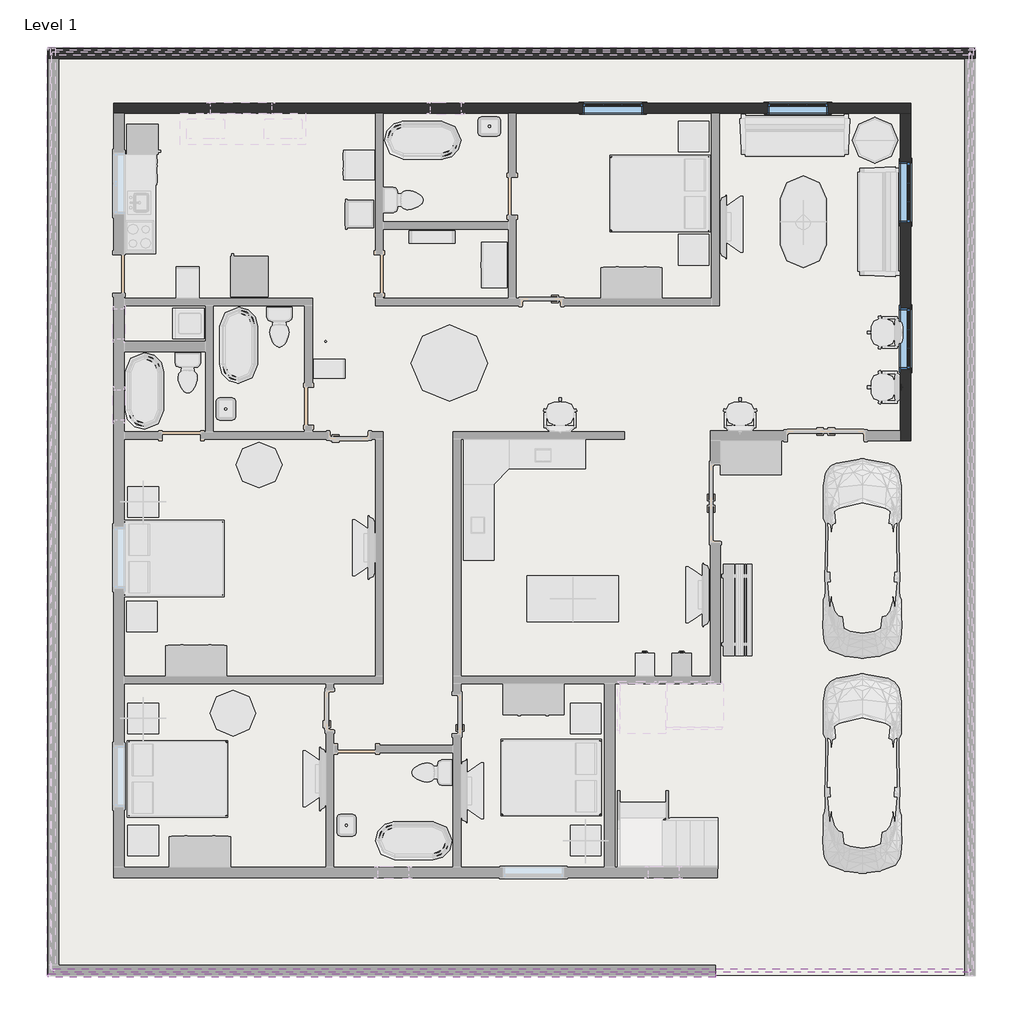
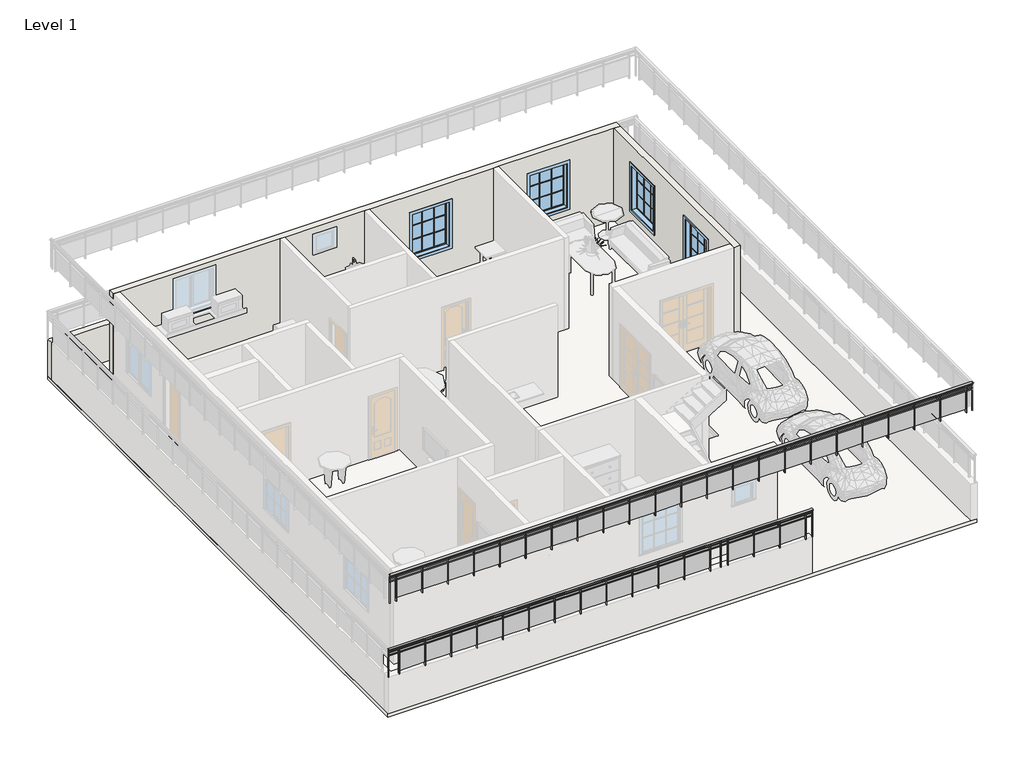
# One storey, part 2 of 6: 4 windows, 3 walls, 2 railings, 1 slab.
"""IFC4 building model written with IfcOpenShell, lengths in millimetres."""

from ifc_helpers import new_model, si_unit, point, frame, origin, place, context, project, spatial, polyline, ellipse_curve, trimmed, outline, extrude, faceted_brep, transform, mapped, element, save
from ifc_brep_helpers import plane_surface, extruded_surface, advanced_brep
from components import window_cfa1ffdd

model = new_model("IFC4")

# Units and contexts
model_context = context("Model", 3, world=origin())
ifc_project = project(units=[si_unit("LENGTHUNIT", "METRE", prefix="MILLI")], contexts=[model_context])

# Site, building, storey
site = spatial("IfcSite", under=ifc_project)
building = spatial("IfcBuilding", under=site)
storey = spatial("IfcBuildingStorey", under=building, Name="Level 1", Elevation=0.0)

# Railings
placement = place(None, origin())
element("IfcRailing", 1, ObjectType="Glass Panel - Bottom Fill", at=placement, inside=storey, context=model_context, shape_type="SolidModel", body=[
    advanced_brep(
    [(-7889.7402326, -4452.2366944, 2133.6), (-7889.7402326, -4528.4366944, 2133.6), (5419.8597674, -4452.2366944, 2133.6), (5419.8597674, -4528.4366944, 2133.6)],
    [
        (0, 1, ellipse_curve(frame((-7889.7402326, -4490.3366944, 2133.6), z_axis=(-1.0, 0.0, 0.0), x_axis=(0.0, -1.0, 0.0)), 38.1, 28.575)),
        (1, 0, ellipse_curve(frame((-7889.7402326, -4490.3366944, 2133.6), z_axis=(-1.0, 0.0, 0.0), x_axis=(0.0, -1.0, 0.0)), 38.1, 28.575)),
        (2, 3, ellipse_curve(frame((5419.8597674, -4490.3366944, 2133.6), z_axis=(1.0, 0.0, 0.0), x_axis=(0.0, -1.0, 0.0)), 38.1, 28.575)),
        (3, 2, ellipse_curve(frame((5419.8597674, -4490.3366944, 2133.6), z_axis=(1.0, 0.0, 0.0), x_axis=(0.0, -1.0, 0.0)), 38.1, 28.575)),
        (0, 2),
        (3, 1),
    ],
    [
        plane_surface(frame((-7889.7402326, -4490.3366944, 2133.6), z_axis=(-1.0, 0.0, 0.0), x_axis=(0.0, 1.0, 0.0))),
        plane_surface(frame((5419.8597674, -4490.3366944, 2133.6), z_axis=(1.0, 0.0, 0.0), x_axis=(0.0, 1.0, 0.0))),
        extruded_surface(trimmed(ellipse_curve(frame((5419.8597674, -4490.3366944, 2133.6), z_axis=(-1.0, 0.0, 0.0), x_axis=(0.0, -1.0, 0.0)), 38.1, 28.575), [point((5419.8597674, -4452.2366944, 2133.6))], [point((5419.8597674, -4528.4366944, 2133.6))], True, "CARTESIAN"), (-13309.6, 0.0, 0.0), 13309.6),
        extruded_surface(trimmed(ellipse_curve(frame((5419.8597674, -4490.3366944, 2133.6), z_axis=(-1.0, 0.0, 0.0), x_axis=(0.0, -1.0, 0.0)), 38.1, 28.575), [point((5419.8597674, -4528.4366944, 2133.6))], [point((5419.8597674, -4452.2366944, 2133.6))], True, "CARTESIAN"), (-13309.6, 0.0, 0.0), 13309.6),
    ],
    [
        (0, [[1, 2]]),
        (1, [[3, 4]]),
        (2, [[-1, 5, -4, 6]]),
        (3, [[-2, -6, -3, -5]]),
    ],
),
    extrude(outline(polyline([(-7889.7402326, -4503.0366944), (-7889.7402326, -4477.6366944), (5419.8597674, -4477.6366944), (5419.8597674, -4503.0366944), (-7889.7402326, -4503.0366944)])), frame((0.0, 0.0, 2019.3), z_axis=(0.0, 0.0, 1.0), x_axis=(1.0, 0.0, 0.0)), (0.0, 0.0, 1.0), 25.4),
    extrude(outline(polyline([(-7889.7402326, -4503.0366944), (-7889.7402326, -4477.6366944), (5419.8597674, -4477.6366944), (5419.8597674, -4503.0366944), (-7889.7402326, -4503.0366944)])), frame((0.0, 0.0, 1917.7), z_axis=(0.0, 0.0, 1.0), x_axis=(1.0, 0.0, 0.0)), (0.0, 0.0, 1.0), 25.4),
    extrude(outline(polyline([(5197.6097674, -4515.7366944), (5197.6097674, -4464.9366944), (5210.3097674, -4464.9366944), (5210.3097674, -4515.7366944), (5197.6097674, -4515.7366944)])), frame((0.0, 0.0, 1219.2), z_axis=(0.0, 0.0, 1.0), x_axis=(1.0, 0.0, 0.0)), (0.0, 0.0, 1.0), 885.6788223),
    extrude(outline(polyline([(4391.1597674, -4483.8015374), (5203.9597674, -4483.8015374), (5203.9597674, -4490.1515374), (4391.1597674, -4490.1515374), (4391.1597674, -4483.8015374)])), frame((0.0, 0.0, 1320.8), z_axis=(0.0, 0.0, 1.0), x_axis=(1.0, 0.0, 0.0)), (0.0, 0.0, 1.0), 596.9),
    extrude(outline(polyline([(4384.8097674, -4515.7366944), (4384.8097674, -4464.9366944), (4397.5097674, -4464.9366944), (4397.5097674, -4515.7366944), (4384.8097674, -4515.7366944)])), frame((0.0, 0.0, 1219.2), z_axis=(0.0, 0.0, 1.0), x_axis=(1.0, 0.0, 0.0)), (0.0, 0.0, 1.0), 885.6788223),
    extrude(outline(polyline([(3578.3597674, -4483.8015374), (4391.1597674, -4483.8015374), (4391.1597674, -4490.1515374), (3578.3597674, -4490.1515374), (3578.3597674, -4483.8015374)])), frame((0.0, 0.0, 1320.8), z_axis=(0.0, 0.0, 1.0), x_axis=(1.0, 0.0, 0.0)), (0.0, 0.0, 1.0), 596.9),
    extrude(outline(polyline([(3572.0097674, -4515.7366944), (3572.0097674, -4464.9366944), (3584.7097674, -4464.9366944), (3584.7097674, -4515.7366944), (3572.0097674, -4515.7366944)])), frame((0.0, 0.0, 1219.2), z_axis=(0.0, 0.0, 1.0), x_axis=(1.0, 0.0, 0.0)), (0.0, 0.0, 1.0), 885.6788223),
    extrude(outline(polyline([(2765.5597674, -4483.8015374), (3578.3597674, -4483.8015374), (3578.3597674, -4490.1515374), (2765.5597674, -4490.1515374), (2765.5597674, -4483.8015374)])), frame((0.0, 0.0, 1320.8), z_axis=(0.0, 0.0, 1.0), x_axis=(1.0, 0.0, 0.0)), (0.0, 0.0, 1.0), 596.9),
    extrude(outline(polyline([(2759.2097674, -4515.7366944), (2759.2097674, -4464.9366944), (2771.9097674, -4464.9366944), (2771.9097674, -4515.7366944), (2759.2097674, -4515.7366944)])), frame((0.0, 0.0, 1219.2), z_axis=(0.0, 0.0, 1.0), x_axis=(1.0, 0.0, 0.0)), (0.0, 0.0, 1.0), 885.6788223),
    extrude(outline(polyline([(2200.4097674, -4515.7366944), (2200.4097674, -4464.9366944), (2213.1097674, -4464.9366944), (2213.1097674, -4515.7366944), (2200.4097674, -4515.7366944)])), frame((0.0, 0.0, 1219.2), z_axis=(0.0, 0.0, 1.0), x_axis=(1.0, 0.0, 0.0)), (0.0, 0.0, 1.0), 885.6788223),
    extrude(outline(polyline([(1393.9597674, -4483.8015374), (2206.7597674, -4483.8015374), (2206.7597674, -4490.1515374), (1393.9597674, -4490.1515374), (1393.9597674, -4483.8015374)])), frame((0.0, 0.0, 1320.8), z_axis=(0.0, 0.0, 1.0), x_axis=(1.0, 0.0, 0.0)), (0.0, 0.0, 1.0), 596.9),
    extrude(outline(polyline([(1387.6097674, -4515.7366944), (1387.6097674, -4464.9366944), (1400.3097674, -4464.9366944), (1400.3097674, -4515.7366944), (1387.6097674, -4515.7366944)])), frame((0.0, 0.0, 1219.2), z_axis=(0.0, 0.0, 1.0), x_axis=(1.0, 0.0, 0.0)), (0.0, 0.0, 1.0), 885.6788223),
    extrude(outline(polyline([(581.1597674, -4483.8015374), (1393.9597674, -4483.8015374), (1393.9597674, -4490.1515374), (581.1597674, -4490.1515374), (581.1597674, -4483.8015374)])), frame((0.0, 0.0, 1320.8), z_axis=(0.0, 0.0, 1.0), x_axis=(1.0, 0.0, 0.0)), (0.0, 0.0, 1.0), 596.9),
    extrude(outline(polyline([(574.8097674, -4515.7366944), (574.8097674, -4464.9366944), (587.5097674, -4464.9366944), (587.5097674, -4515.7366944), (574.8097674, -4515.7366944)])), frame((0.0, 0.0, 1219.2), z_axis=(0.0, 0.0, 1.0), x_axis=(1.0, 0.0, 0.0)), (0.0, 0.0, 1.0), 885.6788223),
    extrude(outline(polyline([(-231.6402326, -4483.8015374), (581.1597674, -4483.8015374), (581.1597674, -4490.1515374), (-231.6402326, -4490.1515374), (-231.6402326, -4483.8015374)])), frame((0.0, 0.0, 1320.8), z_axis=(0.0, 0.0, 1.0), x_axis=(1.0, 0.0, 0.0)), (0.0, 0.0, 1.0), 596.9),
    extrude(outline(polyline([(-237.9902326, -4515.7366944), (-237.9902326, -4464.9366944), (-225.2902326, -4464.9366944), (-225.2902326, -4515.7366944), (-237.9902326, -4515.7366944)])), frame((0.0, 0.0, 1219.2), z_axis=(0.0, 0.0, 1.0), x_axis=(1.0, 0.0, 0.0)), (0.0, 0.0, 1.0), 885.6788223),
    extrude(outline(polyline([(-1044.4402326, -4483.8015374), (-231.6402326, -4483.8015374), (-231.6402326, -4490.1515374), (-1044.4402326, -4490.1515374), (-1044.4402326, -4483.8015374)])), frame((0.0, 0.0, 1320.8), z_axis=(0.0, 0.0, 1.0), x_axis=(1.0, 0.0, 0.0)), (0.0, 0.0, 1.0), 596.9),
    extrude(outline(polyline([(-1050.7902326, -4515.7366944), (-1050.7902326, -4464.9366944), (-1038.0902326, -4464.9366944), (-1038.0902326, -4515.7366944), (-1050.7902326, -4515.7366944)])), frame((0.0, 0.0, 1219.2), z_axis=(0.0, 0.0, 1.0), x_axis=(1.0, 0.0, 0.0)), (0.0, 0.0, 1.0), 885.6788223),
    extrude(outline(polyline([(-1857.2402326, -4483.8015374), (-1044.4402326, -4483.8015374), (-1044.4402326, -4490.1515374), (-1857.2402326, -4490.1515374), (-1857.2402326, -4483.8015374)])), frame((0.0, 0.0, 1320.8), z_axis=(0.0, 0.0, 1.0), x_axis=(1.0, 0.0, 0.0)), (0.0, 0.0, 1.0), 596.9),
    extrude(outline(polyline([(-1863.5902326, -4515.7366944), (-1863.5902326, -4464.9366944), (-1850.8902326, -4464.9366944), (-1850.8902326, -4515.7366944), (-1863.5902326, -4515.7366944)])), frame((0.0, 0.0, 1219.2), z_axis=(0.0, 0.0, 1.0), x_axis=(1.0, 0.0, 0.0)), (0.0, 0.0, 1.0), 885.6788223),
    extrude(outline(polyline([(-2670.0402326, -4483.8015374), (-1857.2402326, -4483.8015374), (-1857.2402326, -4490.1515374), (-2670.0402326, -4490.1515374), (-2670.0402326, -4483.8015374)])), frame((0.0, 0.0, 1320.8), z_axis=(0.0, 0.0, 1.0), x_axis=(1.0, 0.0, 0.0)), (0.0, 0.0, 1.0), 596.9),
    extrude(outline(polyline([(-2676.3902326, -4515.7366944), (-2676.3902326, -4464.9366944), (-2663.6902326, -4464.9366944), (-2663.6902326, -4515.7366944), (-2676.3902326, -4515.7366944)])), frame((0.0, 0.0, 1219.2), z_axis=(0.0, 0.0, 1.0), x_axis=(1.0, 0.0, 0.0)), (0.0, 0.0, 1.0), 885.6788223),
    extrude(outline(polyline([(-3482.8402326, -4483.8015374), (-2670.0402326, -4483.8015374), (-2670.0402326, -4490.1515374), (-3482.8402326, -4490.1515374), (-3482.8402326, -4483.8015374)])), frame((0.0, 0.0, 1320.8), z_axis=(0.0, 0.0, 1.0), x_axis=(1.0, 0.0, 0.0)), (0.0, 0.0, 1.0), 596.9),
    extrude(outline(polyline([(-3489.1902326, -4515.7366944), (-3489.1902326, -4464.9366944), (-3476.4902326, -4464.9366944), (-3476.4902326, -4515.7366944), (-3489.1902326, -4515.7366944)])), frame((0.0, 0.0, 1219.2), z_axis=(0.0, 0.0, 1.0), x_axis=(1.0, 0.0, 0.0)), (0.0, 0.0, 1.0), 885.6788223),
    extrude(outline(polyline([(-4295.6402326, -4483.8015374), (-3482.8402326, -4483.8015374), (-3482.8402326, -4490.1515374), (-4295.6402326, -4490.1515374), (-4295.6402326, -4483.8015374)])), frame((0.0, 0.0, 1320.8), z_axis=(0.0, 0.0, 1.0), x_axis=(1.0, 0.0, 0.0)), (0.0, 0.0, 1.0), 596.9),
    extrude(outline(polyline([(-4301.9902326, -4515.7366944), (-4301.9902326, -4464.9366944), (-4289.2902326, -4464.9366944), (-4289.2902326, -4515.7366944), (-4301.9902326, -4515.7366944)])), frame((0.0, 0.0, 1219.2), z_axis=(0.0, 0.0, 1.0), x_axis=(1.0, 0.0, 0.0)), (0.0, 0.0, 1.0), 885.6788223),
    extrude(outline(polyline([(-5108.4402326, -4483.8015374), (-4295.6402326, -4483.8015374), (-4295.6402326, -4490.1515374), (-5108.4402326, -4490.1515374), (-5108.4402326, -4483.8015374)])), frame((0.0, 0.0, 1320.8), z_axis=(0.0, 0.0, 1.0), x_axis=(1.0, 0.0, 0.0)), (0.0, 0.0, 1.0), 596.9),
    extrude(outline(polyline([(-5114.7902326, -4515.7366944), (-5114.7902326, -4464.9366944), (-5102.0902326, -4464.9366944), (-5102.0902326, -4515.7366944), (-5114.7902326, -4515.7366944)])), frame((0.0, 0.0, 1219.2), z_axis=(0.0, 0.0, 1.0), x_axis=(1.0, 0.0, 0.0)), (0.0, 0.0, 1.0), 885.6788223),
    extrude(outline(polyline([(-5921.2402326, -4483.8015374), (-5108.4402326, -4483.8015374), (-5108.4402326, -4490.1515374), (-5921.2402326, -4490.1515374), (-5921.2402326, -4483.8015374)])), frame((0.0, 0.0, 1320.8), z_axis=(0.0, 0.0, 1.0), x_axis=(1.0, 0.0, 0.0)), (0.0, 0.0, 1.0), 596.9),
    extrude(outline(polyline([(-5927.5902326, -4515.7366944), (-5927.5902326, -4464.9366944), (-5914.8902326, -4464.9366944), (-5914.8902326, -4515.7366944), (-5927.5902326, -4515.7366944)])), frame((0.0, 0.0, 1219.2), z_axis=(0.0, 0.0, 1.0), x_axis=(1.0, 0.0, 0.0)), (0.0, 0.0, 1.0), 885.6788223),
    extrude(outline(polyline([(-6734.0402326, -4483.8015374), (-5921.2402326, -4483.8015374), (-5921.2402326, -4490.1515374), (-6734.0402326, -4490.1515374), (-6734.0402326, -4483.8015374)])), frame((0.0, 0.0, 1320.8), z_axis=(0.0, 0.0, 1.0), x_axis=(1.0, 0.0, 0.0)), (0.0, 0.0, 1.0), 596.9),
    extrude(outline(polyline([(-6740.3902326, -4515.7366944), (-6740.3902326, -4464.9366944), (-6727.6902326, -4464.9366944), (-6727.6902326, -4515.7366944), (-6740.3902326, -4515.7366944)])), frame((0.0, 0.0, 1219.2), z_axis=(0.0, 0.0, 1.0), x_axis=(1.0, 0.0, 0.0)), (0.0, 0.0, 1.0), 885.6788223),
    extrude(outline(polyline([(-7546.8402326, -4483.8015374), (-6734.0402326, -4483.8015374), (-6734.0402326, -4490.1515374), (-7546.8402326, -4490.1515374), (-7546.8402326, -4483.8015374)])), frame((0.0, 0.0, 1320.8), z_axis=(0.0, 0.0, 1.0), x_axis=(1.0, 0.0, 0.0)), (0.0, 0.0, 1.0), 596.9),
    extrude(outline(polyline([(-7553.1902326, -4515.7366944), (-7553.1902326, -4464.9366944), (-7540.4902326, -4464.9366944), (-7540.4902326, -4515.7366944), (-7553.1902326, -4515.7366944)])), frame((0.0, 0.0, 1219.2), z_axis=(0.0, 0.0, 1.0), x_axis=(1.0, 0.0, 0.0)), (0.0, 0.0, 1.0), 885.6788223),
    extrude(outline(polyline([(2540.1347674, -4499.8616944), (2540.1347674, -4480.8116944), (2559.1847674, -4480.8116944), (2559.1847674, -4499.8616944), (2540.1347674, -4499.8616944)])), frame((0.0, 0.0, 1219.2), z_axis=(0.0, 0.0, 1.0), x_axis=(1.0, 0.0, 0.0)), (0.0, 0.0, 1.0), 885.6788223),
    extrude(outline(polyline([(5407.1597674, -4499.8616944), (5407.1597674, -4480.8116944), (5426.2097674, -4480.8116944), (5426.2097674, -4499.8616944), (5407.1597674, -4499.8616944)])), frame((0.0, 0.0, 1219.2), z_axis=(0.0, 0.0, 1.0), x_axis=(1.0, 0.0, 0.0)), (0.0, 0.0, 1.0), 885.6788223),
    extrude(outline(polyline([(-7896.0902326, -4499.8616944), (-7896.0902326, -4480.8116944), (-7877.0402326, -4480.8116944), (-7877.0402326, -4499.8616944), (-7896.0902326, -4499.8616944)])), frame((0.0, 0.0, 1219.2), z_axis=(0.0, 0.0, 1.0), x_axis=(1.0, 0.0, 0.0)), (0.0, 0.0, 1.0), 885.6788223),
])
element("IfcRailing", 2, ObjectType="Glass Panel - Bottom Fill", at=placement, inside=storey, context=model_context, shape_type="SolidModel", body=[
    advanced_brep(
    [(-7788.1402326, -4350.6366944, 4495.8), (-7788.1402326, -4426.8366944, 4495.8), (10499.8597674, -4350.6366944, 4495.8), (10499.8597674, -4426.8366944, 4495.8)],
    [
        (0, 1, ellipse_curve(frame((-7788.1402326, -4388.7366944, 4495.8), z_axis=(-1.0, 0.0, 0.0), x_axis=(0.0, -1.0, 0.0)), 38.1, 28.575)),
        (1, 0, ellipse_curve(frame((-7788.1402326, -4388.7366944, 4495.8), z_axis=(-1.0, 0.0, 0.0), x_axis=(0.0, -1.0, 0.0)), 38.1, 28.575)),
        (2, 3, ellipse_curve(frame((10499.8597674, -4388.7366944, 4495.8), z_axis=(1.0, 0.0, 0.0), x_axis=(0.0, -1.0, 0.0)), 38.1, 28.575)),
        (3, 2, ellipse_curve(frame((10499.8597674, -4388.7366944, 4495.8), z_axis=(1.0, 0.0, 0.0), x_axis=(0.0, -1.0, 0.0)), 38.1, 28.575)),
        (0, 2),
        (3, 1),
    ],
    [
        plane_surface(frame((-7788.1402326, -4388.7366944, 4495.8), z_axis=(-1.0, 0.0, 0.0), x_axis=(0.0, 1.0, 0.0))),
        plane_surface(frame((10499.8597674, -4388.7366944, 4495.8), z_axis=(1.0, 0.0, 0.0), x_axis=(0.0, 1.0, 0.0))),
        extruded_surface(trimmed(ellipse_curve(frame((10499.8597674, -4388.7366944, 4495.8), z_axis=(-1.0, 0.0, 0.0), x_axis=(0.0, -1.0, 0.0)), 38.1, 28.575), [point((10499.8597674, -4350.6366944, 4495.8))], [point((10499.8597674, -4426.8366944, 4495.8))], True, "CARTESIAN"), (-18288.0, 0.0, 0.0), 18288.0),
        extruded_surface(trimmed(ellipse_curve(frame((10499.8597674, -4388.7366944, 4495.8), z_axis=(-1.0, 0.0, 0.0), x_axis=(0.0, -1.0, 0.0)), 38.1, 28.575), [point((10499.8597674, -4426.8366944, 4495.8))], [point((10499.8597674, -4350.6366944, 4495.8))], True, "CARTESIAN"), (-18288.0, 0.0, 0.0), 18288.0),
    ],
    [
        (0, [[1, 2]]),
        (1, [[3, 4]]),
        (2, [[-1, 5, -4, 6]]),
        (3, [[-2, -6, -3, -5]]),
    ],
),
    extrude(outline(polyline([(-7788.1402326, -4401.4366944), (-7788.1402326, -4376.0366944), (10499.8597674, -4376.0366944), (10499.8597674, -4401.4366944), (-7788.1402326, -4401.4366944)])), frame((0.0, 0.0, 4381.5), z_axis=(0.0, 0.0, 1.0), x_axis=(1.0, 0.0, 0.0)), (0.0, 0.0, 1.0), 25.4),
    extrude(outline(polyline([(-7788.1402326, -4401.4366944), (-7788.1402326, -4376.0366944), (10499.8597674, -4376.0366944), (10499.8597674, -4401.4366944), (-7788.1402326, -4401.4366944)])), frame((0.0, 0.0, 4279.9), z_axis=(0.0, 0.0, 1.0), x_axis=(1.0, 0.0, 0.0)), (0.0, 0.0, 1.0), 25.4),
    extrude(outline(polyline([(10290.3097674, -4414.1366944), (10290.3097674, -4363.3366944), (10303.0097674, -4363.3366944), (10303.0097674, -4414.1366944), (10290.3097674, -4414.1366944)])), frame((0.0, 0.0, 3581.4), z_axis=(0.0, 0.0, 1.0), x_axis=(1.0, 0.0, 0.0)), (0.0, 0.0, 1.0), 885.6788223),
    extrude(outline(polyline([(9483.8597674, -4382.2015374), (10296.6597674, -4382.2015374), (10296.6597674, -4388.5515374), (9483.8597674, -4388.5515374), (9483.8597674, -4382.2015374)])), frame((0.0, 0.0, 3683.0), z_axis=(0.0, 0.0, 1.0), x_axis=(1.0, 0.0, 0.0)), (0.0, 0.0, 1.0), 596.9),
    extrude(outline(polyline([(9477.5097674, -4414.1366944), (9477.5097674, -4363.3366944), (9490.2097674, -4363.3366944), (9490.2097674, -4414.1366944), (9477.5097674, -4414.1366944)])), frame((0.0, 0.0, 3581.4), z_axis=(0.0, 0.0, 1.0), x_axis=(1.0, 0.0, 0.0)), (0.0, 0.0, 1.0), 885.6788223),
    extrude(outline(polyline([(8671.0597674, -4382.2015374), (9483.8597674, -4382.2015374), (9483.8597674, -4388.5515374), (8671.0597674, -4388.5515374), (8671.0597674, -4382.2015374)])), frame((0.0, 0.0, 3683.0), z_axis=(0.0, 0.0, 1.0), x_axis=(1.0, 0.0, 0.0)), (0.0, 0.0, 1.0), 596.9),
    extrude(outline(polyline([(8664.7097674, -4414.1366944), (8664.7097674, -4363.3366944), (8677.4097674, -4363.3366944), (8677.4097674, -4414.1366944), (8664.7097674, -4414.1366944)])), frame((0.0, 0.0, 3581.4), z_axis=(0.0, 0.0, 1.0), x_axis=(1.0, 0.0, 0.0)), (0.0, 0.0, 1.0), 885.6788223),
    extrude(outline(polyline([(7858.2597674, -4382.2015374), (8671.0597674, -4382.2015374), (8671.0597674, -4388.5515374), (7858.2597674, -4388.5515374), (7858.2597674, -4382.2015374)])), frame((0.0, 0.0, 3683.0), z_axis=(0.0, 0.0, 1.0), x_axis=(1.0, 0.0, 0.0)), (0.0, 0.0, 1.0), 596.9),
    extrude(outline(polyline([(7851.9097674, -4414.1366944), (7851.9097674, -4363.3366944), (7864.6097674, -4363.3366944), (7864.6097674, -4414.1366944), (7851.9097674, -4414.1366944)])), frame((0.0, 0.0, 3581.4), z_axis=(0.0, 0.0, 1.0), x_axis=(1.0, 0.0, 0.0)), (0.0, 0.0, 1.0), 885.6788223),
    extrude(outline(polyline([(7045.4597674, -4382.2015374), (7858.2597674, -4382.2015374), (7858.2597674, -4388.5515374), (7045.4597674, -4388.5515374), (7045.4597674, -4382.2015374)])), frame((0.0, 0.0, 3683.0), z_axis=(0.0, 0.0, 1.0), x_axis=(1.0, 0.0, 0.0)), (0.0, 0.0, 1.0), 596.9),
    extrude(outline(polyline([(7039.1097674, -4414.1366944), (7039.1097674, -4363.3366944), (7051.8097674, -4363.3366944), (7051.8097674, -4414.1366944), (7039.1097674, -4414.1366944)])), frame((0.0, 0.0, 3581.4), z_axis=(0.0, 0.0, 1.0), x_axis=(1.0, 0.0, 0.0)), (0.0, 0.0, 1.0), 885.6788223),
    extrude(outline(polyline([(6232.6597674, -4382.2015374), (7045.4597674, -4382.2015374), (7045.4597674, -4388.5515374), (6232.6597674, -4388.5515374), (6232.6597674, -4382.2015374)])), frame((0.0, 0.0, 3683.0), z_axis=(0.0, 0.0, 1.0), x_axis=(1.0, 0.0, 0.0)), (0.0, 0.0, 1.0), 596.9),
    extrude(outline(polyline([(6226.3097674, -4414.1366944), (6226.3097674, -4363.3366944), (6239.0097674, -4363.3366944), (6239.0097674, -4414.1366944), (6226.3097674, -4414.1366944)])), frame((0.0, 0.0, 3581.4), z_axis=(0.0, 0.0, 1.0), x_axis=(1.0, 0.0, 0.0)), (0.0, 0.0, 1.0), 885.6788223),
    extrude(outline(polyline([(5419.8597674, -4382.2015374), (6232.6597674, -4382.2015374), (6232.6597674, -4388.5515374), (5419.8597674, -4388.5515374), (5419.8597674, -4382.2015374)])), frame((0.0, 0.0, 3683.0), z_axis=(0.0, 0.0, 1.0), x_axis=(1.0, 0.0, 0.0)), (0.0, 0.0, 1.0), 596.9),
    extrude(outline(polyline([(5413.5097674, -4414.1366944), (5413.5097674, -4363.3366944), (5426.2097674, -4363.3366944), (5426.2097674, -4414.1366944), (5413.5097674, -4414.1366944)])), frame((0.0, 0.0, 3581.4), z_axis=(0.0, 0.0, 1.0), x_axis=(1.0, 0.0, 0.0)), (0.0, 0.0, 1.0), 885.6788223),
    extrude(outline(polyline([(4607.0597674, -4382.2015374), (5419.8597674, -4382.2015374), (5419.8597674, -4388.5515374), (4607.0597674, -4388.5515374), (4607.0597674, -4382.2015374)])), frame((0.0, 0.0, 3683.0), z_axis=(0.0, 0.0, 1.0), x_axis=(1.0, 0.0, 0.0)), (0.0, 0.0, 1.0), 596.9),
    extrude(outline(polyline([(4600.7097674, -4414.1366944), (4600.7097674, -4363.3366944), (4613.4097674, -4363.3366944), (4613.4097674, -4414.1366944), (4600.7097674, -4414.1366944)])), frame((0.0, 0.0, 3581.4), z_axis=(0.0, 0.0, 1.0), x_axis=(1.0, 0.0, 0.0)), (0.0, 0.0, 1.0), 885.6788223),
    extrude(outline(polyline([(3794.2597674, -4382.2015374), (4607.0597674, -4382.2015374), (4607.0597674, -4388.5515374), (3794.2597674, -4388.5515374), (3794.2597674, -4382.2015374)])), frame((0.0, 0.0, 3683.0), z_axis=(0.0, 0.0, 1.0), x_axis=(1.0, 0.0, 0.0)), (0.0, 0.0, 1.0), 596.9),
    extrude(outline(polyline([(3787.9097674, -4414.1366944), (3787.9097674, -4363.3366944), (3800.6097674, -4363.3366944), (3800.6097674, -4414.1366944), (3787.9097674, -4414.1366944)])), frame((0.0, 0.0, 3581.4), z_axis=(0.0, 0.0, 1.0), x_axis=(1.0, 0.0, 0.0)), (0.0, 0.0, 1.0), 885.6788223),
    extrude(outline(polyline([(2981.4597674, -4382.2015374), (3794.2597674, -4382.2015374), (3794.2597674, -4388.5515374), (2981.4597674, -4388.5515374), (2981.4597674, -4382.2015374)])), frame((0.0, 0.0, 3683.0), z_axis=(0.0, 0.0, 1.0), x_axis=(1.0, 0.0, 0.0)), (0.0, 0.0, 1.0), 596.9),
    extrude(outline(polyline([(2975.1097674, -4414.1366944), (2975.1097674, -4363.3366944), (2987.8097674, -4363.3366944), (2987.8097674, -4414.1366944), (2975.1097674, -4414.1366944)])), frame((0.0, 0.0, 3581.4), z_axis=(0.0, 0.0, 1.0), x_axis=(1.0, 0.0, 0.0)), (0.0, 0.0, 1.0), 885.6788223),
    extrude(outline(polyline([(2168.6597674, -4382.2015374), (2981.4597674, -4382.2015374), (2981.4597674, -4388.5515374), (2168.6597674, -4388.5515374), (2168.6597674, -4382.2015374)])), frame((0.0, 0.0, 3683.0), z_axis=(0.0, 0.0, 1.0), x_axis=(1.0, 0.0, 0.0)), (0.0, 0.0, 1.0), 596.9),
    extrude(outline(polyline([(2162.3097674, -4414.1366944), (2162.3097674, -4363.3366944), (2175.0097674, -4363.3366944), (2175.0097674, -4414.1366944), (2162.3097674, -4414.1366944)])), frame((0.0, 0.0, 3581.4), z_axis=(0.0, 0.0, 1.0), x_axis=(1.0, 0.0, 0.0)), (0.0, 0.0, 1.0), 885.6788223),
    extrude(outline(polyline([(1355.8597674, -4382.2015374), (2168.6597674, -4382.2015374), (2168.6597674, -4388.5515374), (1355.8597674, -4388.5515374), (1355.8597674, -4382.2015374)])), frame((0.0, 0.0, 3683.0), z_axis=(0.0, 0.0, 1.0), x_axis=(1.0, 0.0, 0.0)), (0.0, 0.0, 1.0), 596.9),
    extrude(outline(polyline([(1349.5097674, -4414.1366944), (1349.5097674, -4363.3366944), (1362.2097674, -4363.3366944), (1362.2097674, -4414.1366944), (1349.5097674, -4414.1366944)])), frame((0.0, 0.0, 3581.4), z_axis=(0.0, 0.0, 1.0), x_axis=(1.0, 0.0, 0.0)), (0.0, 0.0, 1.0), 885.6788223),
    extrude(outline(polyline([(543.0597674, -4382.2015374), (1355.8597674, -4382.2015374), (1355.8597674, -4388.5515374), (543.0597674, -4388.5515374), (543.0597674, -4382.2015374)])), frame((0.0, 0.0, 3683.0), z_axis=(0.0, 0.0, 1.0), x_axis=(1.0, 0.0, 0.0)), (0.0, 0.0, 1.0), 596.9),
    extrude(outline(polyline([(536.7097674, -4414.1366944), (536.7097674, -4363.3366944), (549.4097674, -4363.3366944), (549.4097674, -4414.1366944), (536.7097674, -4414.1366944)])), frame((0.0, 0.0, 3581.4), z_axis=(0.0, 0.0, 1.0), x_axis=(1.0, 0.0, 0.0)), (0.0, 0.0, 1.0), 885.6788223),
    extrude(outline(polyline([(-269.7402326, -4382.2015374), (543.0597674, -4382.2015374), (543.0597674, -4388.5515374), (-269.7402326, -4388.5515374), (-269.7402326, -4382.2015374)])), frame((0.0, 0.0, 3683.0), z_axis=(0.0, 0.0, 1.0), x_axis=(1.0, 0.0, 0.0)), (0.0, 0.0, 1.0), 596.9),
    extrude(outline(polyline([(-276.0902326, -4414.1366944), (-276.0902326, -4363.3366944), (-263.3902326, -4363.3366944), (-263.3902326, -4414.1366944), (-276.0902326, -4414.1366944)])), frame((0.0, 0.0, 3581.4), z_axis=(0.0, 0.0, 1.0), x_axis=(1.0, 0.0, 0.0)), (0.0, 0.0, 1.0), 885.6788223),
    extrude(outline(polyline([(-1082.5402326, -4382.2015374), (-269.7402326, -4382.2015374), (-269.7402326, -4388.5515374), (-1082.5402326, -4388.5515374), (-1082.5402326, -4382.2015374)])), frame((0.0, 0.0, 3683.0), z_axis=(0.0, 0.0, 1.0), x_axis=(1.0, 0.0, 0.0)), (0.0, 0.0, 1.0), 596.9),
    extrude(outline(polyline([(-1088.8902326, -4414.1366944), (-1088.8902326, -4363.3366944), (-1076.1902326, -4363.3366944), (-1076.1902326, -4414.1366944), (-1088.8902326, -4414.1366944)])), frame((0.0, 0.0, 3581.4), z_axis=(0.0, 0.0, 1.0), x_axis=(1.0, 0.0, 0.0)), (0.0, 0.0, 1.0), 885.6788223),
    extrude(outline(polyline([(-1895.3402326, -4382.2015374), (-1082.5402326, -4382.2015374), (-1082.5402326, -4388.5515374), (-1895.3402326, -4388.5515374), (-1895.3402326, -4382.2015374)])), frame((0.0, 0.0, 3683.0), z_axis=(0.0, 0.0, 1.0), x_axis=(1.0, 0.0, 0.0)), (0.0, 0.0, 1.0), 596.9),
    extrude(outline(polyline([(-1901.6902326, -4414.1366944), (-1901.6902326, -4363.3366944), (-1888.9902326, -4363.3366944), (-1888.9902326, -4414.1366944), (-1901.6902326, -4414.1366944)])), frame((0.0, 0.0, 3581.4), z_axis=(0.0, 0.0, 1.0), x_axis=(1.0, 0.0, 0.0)), (0.0, 0.0, 1.0), 885.6788223),
    extrude(outline(polyline([(-2708.1402326, -4382.2015374), (-1895.3402326, -4382.2015374), (-1895.3402326, -4388.5515374), (-2708.1402326, -4388.5515374), (-2708.1402326, -4382.2015374)])), frame((0.0, 0.0, 3683.0), z_axis=(0.0, 0.0, 1.0), x_axis=(1.0, 0.0, 0.0)), (0.0, 0.0, 1.0), 596.9),
    extrude(outline(polyline([(-2714.4902326, -4414.1366944), (-2714.4902326, -4363.3366944), (-2701.7902326, -4363.3366944), (-2701.7902326, -4414.1366944), (-2714.4902326, -4414.1366944)])), frame((0.0, 0.0, 3581.4), z_axis=(0.0, 0.0, 1.0), x_axis=(1.0, 0.0, 0.0)), (0.0, 0.0, 1.0), 885.6788223),
    extrude(outline(polyline([(-3520.9402326, -4382.2015374), (-2708.1402326, -4382.2015374), (-2708.1402326, -4388.5515374), (-3520.9402326, -4388.5515374), (-3520.9402326, -4382.2015374)])), frame((0.0, 0.0, 3683.0), z_axis=(0.0, 0.0, 1.0), x_axis=(1.0, 0.0, 0.0)), (0.0, 0.0, 1.0), 596.9),
    extrude(outline(polyline([(-3527.2902326, -4414.1366944), (-3527.2902326, -4363.3366944), (-3514.5902326, -4363.3366944), (-3514.5902326, -4414.1366944), (-3527.2902326, -4414.1366944)])), frame((0.0, 0.0, 3581.4), z_axis=(0.0, 0.0, 1.0), x_axis=(1.0, 0.0, 0.0)), (0.0, 0.0, 1.0), 885.6788223),
    extrude(outline(polyline([(-4333.7402326, -4382.2015374), (-3520.9402326, -4382.2015374), (-3520.9402326, -4388.5515374), (-4333.7402326, -4388.5515374), (-4333.7402326, -4382.2015374)])), frame((0.0, 0.0, 3683.0), z_axis=(0.0, 0.0, 1.0), x_axis=(1.0, 0.0, 0.0)), (0.0, 0.0, 1.0), 596.9),
    extrude(outline(polyline([(-4340.0902326, -4414.1366944), (-4340.0902326, -4363.3366944), (-4327.3902326, -4363.3366944), (-4327.3902326, -4414.1366944), (-4340.0902326, -4414.1366944)])), frame((0.0, 0.0, 3581.4), z_axis=(0.0, 0.0, 1.0), x_axis=(1.0, 0.0, 0.0)), (0.0, 0.0, 1.0), 885.6788223),
    extrude(outline(polyline([(-5146.5402326, -4382.2015374), (-4333.7402326, -4382.2015374), (-4333.7402326, -4388.5515374), (-5146.5402326, -4388.5515374), (-5146.5402326, -4382.2015374)])), frame((0.0, 0.0, 3683.0), z_axis=(0.0, 0.0, 1.0), x_axis=(1.0, 0.0, 0.0)), (0.0, 0.0, 1.0), 596.9),
    extrude(outline(polyline([(-5152.8902326, -4414.1366944), (-5152.8902326, -4363.3366944), (-5140.1902326, -4363.3366944), (-5140.1902326, -4414.1366944), (-5152.8902326, -4414.1366944)])), frame((0.0, 0.0, 3581.4), z_axis=(0.0, 0.0, 1.0), x_axis=(1.0, 0.0, 0.0)), (0.0, 0.0, 1.0), 885.6788223),
    extrude(outline(polyline([(-5959.3402326, -4382.2015374), (-5146.5402326, -4382.2015374), (-5146.5402326, -4388.5515374), (-5959.3402326, -4388.5515374), (-5959.3402326, -4382.2015374)])), frame((0.0, 0.0, 3683.0), z_axis=(0.0, 0.0, 1.0), x_axis=(1.0, 0.0, 0.0)), (0.0, 0.0, 1.0), 596.9),
    extrude(outline(polyline([(-5965.6902326, -4414.1366944), (-5965.6902326, -4363.3366944), (-5952.9902326, -4363.3366944), (-5952.9902326, -4414.1366944), (-5965.6902326, -4414.1366944)])), frame((0.0, 0.0, 3581.4), z_axis=(0.0, 0.0, 1.0), x_axis=(1.0, 0.0, 0.0)), (0.0, 0.0, 1.0), 885.6788223),
    extrude(outline(polyline([(-6772.1402326, -4382.2015374), (-5959.3402326, -4382.2015374), (-5959.3402326, -4388.5515374), (-6772.1402326, -4388.5515374), (-6772.1402326, -4382.2015374)])), frame((0.0, 0.0, 3683.0), z_axis=(0.0, 0.0, 1.0), x_axis=(1.0, 0.0, 0.0)), (0.0, 0.0, 1.0), 596.9),
    extrude(outline(polyline([(-6778.4902326, -4414.1366944), (-6778.4902326, -4363.3366944), (-6765.7902326, -4363.3366944), (-6765.7902326, -4414.1366944), (-6778.4902326, -4414.1366944)])), frame((0.0, 0.0, 3581.4), z_axis=(0.0, 0.0, 1.0), x_axis=(1.0, 0.0, 0.0)), (0.0, 0.0, 1.0), 885.6788223),
    extrude(outline(polyline([(-7584.9402326, -4382.2015374), (-6772.1402326, -4382.2015374), (-6772.1402326, -4388.5515374), (-7584.9402326, -4388.5515374), (-7584.9402326, -4382.2015374)])), frame((0.0, 0.0, 3683.0), z_axis=(0.0, 0.0, 1.0), x_axis=(1.0, 0.0, 0.0)), (0.0, 0.0, 1.0), 596.9),
    extrude(outline(polyline([(-7591.2902326, -4414.1366944), (-7591.2902326, -4363.3366944), (-7578.5902326, -4363.3366944), (-7578.5902326, -4414.1366944), (-7591.2902326, -4414.1366944)])), frame((0.0, 0.0, 3581.4), z_axis=(0.0, 0.0, 1.0), x_axis=(1.0, 0.0, 0.0)), (0.0, 0.0, 1.0), 885.6788223),
    extrude(outline(polyline([(10487.1597674, -4398.2616944), (10487.1597674, -4379.2116944), (10506.2097674, -4379.2116944), (10506.2097674, -4398.2616944), (10487.1597674, -4398.2616944)])), frame((0.0, 0.0, 3581.4), z_axis=(0.0, 0.0, 1.0), x_axis=(1.0, 0.0, 0.0)), (0.0, 0.0, 1.0), 885.6788223),
    extrude(outline(polyline([(-7794.4902326, -4398.2616944), (-7794.4902326, -4379.2116944), (-7775.4402326, -4379.2116944), (-7775.4402326, -4398.2616944), (-7794.4902326, -4398.2616944)])), frame((0.0, 0.0, 3581.4), z_axis=(0.0, 0.0, 1.0), x_axis=(1.0, 0.0, 0.0)), (0.0, 0.0, 1.0), 885.6788223),
])

# Slab
element("IfcSlab", 3, ObjectType="LW Concrete on Metal Deck", at=placement, inside=storey, context=model_context, shape_type="SweptSolid", body=[
    extrude(outline(polyline([(-7899.2652326, 14000.8633056), (10588.7597674, 14000.8633056), (10588.7597674, -4487.1616944), (-7899.2652326, -4487.1616944), (-7899.2652326, 14000.8633056)])), frame((0.0, 0.0, -104.775), z_axis=(0.0, 0.0, 1.0), x_axis=(1.0, 0.0, 0.0)), (0.0, 0.0, 1.0), 104.775),
])

# Walls
element("IfcWall", 4, at=placement, inside=storey, context=model_context, shape_type="Brep", body=[
    faceted_brep([(-7889.7402326, 13797.6633056, 0.0), (-7686.5402326, 13797.6633056, 0.0), (10398.2597674, 13797.6633056, 0.0), (10601.4597674, 13797.6633056, 0.0), (10601.4597674, 13797.6633056, 1219.2), (10398.2597674, 13797.6633056, 1219.2), (-7686.5402326, 13797.6633056, 1219.2), (-7889.7402326, 13797.6633056, 1219.2), (-7889.7402326, 14000.8633056, 0.0), (-7889.7402326, 14000.8633056, 1219.2), (10601.4597674, 14000.8633056, 1219.2), (10601.4597674, 14000.8633056, 0.0)], [[[0, 1, 2, 3, 4, 5, 6, 7]], [[8, 9, 10, 11]], [[3, 2, 1, 0, 8, 11]], [[7, 6, 5, 4, 10, 9]], [[4, 3, 11, 10]], [[0, 7, 9, 8]]]),
])
element("IfcWall", 5, ObjectType="Generic - 8\"", at=placement, inside=storey, context=model_context, shape_type="Brep", body=[
    faceted_brep([(-6583.5787181, 12704.3758265, 0.0), (-6380.3787181, 12704.3758265, 0.0), (-1361.9402326, 12704.3758265, 0.0), (-1209.5402326, 12704.3758265, 0.0), (1290.4212819, 12704.3758265, 0.0), (1442.8212819, 12704.3758265, 0.0), (5343.6597674, 12704.3758265, 0.0), (5496.0597674, 12704.3758265, 0.0), (9113.6212819, 12704.3758265, 0.0), (9316.8212819, 12704.3758265, 0.0), (9316.8212819, 12704.3758265, 3048.0), (9113.6212819, 12704.3758265, 3048.0), (5496.0597674, 12704.3758265, 3048.0), (5343.6597674, 12704.3758265, 3048.0), (1442.8212819, 12704.3758265, 3048.0), (1290.4212819, 12704.3758265, 3048.0), (-1209.5402326, 12704.3758265, 3048.0), (-1361.9402326, 12704.3758265, 3048.0), (-6380.3787181, 12704.3758265, 3048.0), (-6583.5787181, 12704.3758265, 3048.0), (3982.8212819, 12704.3758265, 2438.4), (3982.8212819, 12704.3758265, 914.4), (2763.6212819, 12704.3758265, 914.4), (2763.6212819, 12704.3758265, 2438.4), (7673.1405246, 12704.3758265, 2438.4), (7673.1405246, 12704.3758265, 914.4), (6453.9405246, 12704.3758265, 914.4), (6453.9405246, 12704.3758265, 2438.4), (-3433.9787181, 12704.3758265, 2844.8), (-3433.9787181, 12704.3758265, 1625.6), (-4653.1787181, 12704.3758265, 1625.6), (-4653.1787181, 12704.3758265, 2844.8), (-264.3594754, 12704.3758265, 2768.6), (345.2405246, 12704.3758265, 2768.6), (345.2405246, 12704.3758265, 2159.0), (-264.3594754, 12704.3758265, 2159.0), (-6583.5787181, 12907.5758265, 0.0), (-6583.5787181, 12907.5758265, 3048.0), (9316.8212819, 12907.5758265, 3048.0), (9316.8212819, 12907.5758265, 0.0), (3982.8212819, 12907.5758265, 2438.4), (2763.6212819, 12907.5758265, 2438.4), (2763.6212819, 12907.5758265, 914.4), (3982.8212819, 12907.5758265, 914.4), (7673.1405246, 12907.5758265, 2438.4), (6453.9405246, 12907.5758265, 2438.4), (6453.9405246, 12907.5758265, 914.4), (7673.1405246, 12907.5758265, 914.4), (-3433.9787181, 12907.5758265, 2844.8), (-4653.1787181, 12907.5758265, 2844.8), (-4653.1787181, 12907.5758265, 1625.6), (-3433.9787181, 12907.5758265, 1625.6), (-264.3594754, 12907.5758265, 2768.6), (-264.3594754, 12907.5758265, 2159.0), (345.2405246, 12907.5758265, 2159.0), (345.2405246, 12907.5758265, 2768.6)], [[[0, 1, 2, 3, 4, 5, 6, 7, 8, 9, 10, 11, 12, 13, 14, 15, 16, 17, 18, 19], [20, 21, 22, 23], [24, 25, 26, 27], [28, 29, 30, 31], [32, 33, 34, 35]], [[36, 37, 38, 39], [40, 41, 42, 43], [44, 45, 46, 47], [48, 49, 50, 51], [52, 53, 54, 55]], [[9, 8, 7, 6, 5, 4, 3, 2, 1, 0, 36, 39]], [[10, 9, 39, 38]], [[0, 19, 37, 36]], [[21, 20, 40, 43]], [[22, 21, 43, 42]], [[23, 22, 42, 41]], [[20, 23, 41, 40]], [[25, 24, 44, 47]], [[26, 25, 47, 46]], [[27, 26, 46, 45]], [[24, 27, 45, 44]], [[29, 28, 48, 51]], [[30, 29, 51, 50]], [[31, 30, 50, 49]], [[28, 31, 49, 48]], [[53, 52, 32, 35]], [[54, 53, 35, 34]], [[55, 54, 34, 33]], [[52, 55, 33, 32]], [[19, 18, 17, 16, 15, 14, 13, 12, 11, 10, 38, 37]]]),
])
element("IfcWall", 6, ObjectType="Generic - 8\"", at=placement, inside=storey, context=model_context, shape_type="Brep", body=[
    faceted_brep([(9113.6212819, 12704.3758265, 0.0), (9113.6212819, 6379.7758265, 0.0), (9113.6212819, 6176.5758265, 0.0), (9113.6212819, 6176.5758265, 3048.0), (9113.6212819, 6379.7758265, 3048.0), (9113.6212819, 12704.3758265, 3048.0), (9113.6212819, 10519.9758265, 2438.4), (9113.6212819, 10519.9758265, 914.4), (9113.6212819, 11739.1758265, 914.4), (9113.6212819, 11739.1758265, 2438.4), (9113.6212819, 7598.9758265, 2438.4), (9113.6212819, 7598.9758265, 914.4), (9113.6212819, 8818.1758265, 914.4), (9113.6212819, 8818.1758265, 2438.4), (9316.8212819, 12704.3758265, 0.0), (9316.8212819, 12704.3758265, 3048.0), (9316.8212819, 6176.5758265, 3048.0), (9316.8212819, 6176.5758265, 0.0), (9316.8212819, 10519.9758265, 2438.4), (9316.8212819, 11739.1758265, 2438.4), (9316.8212819, 11739.1758265, 914.4), (9316.8212819, 10519.9758265, 914.4), (9316.8212819, 7598.9758265, 2438.4), (9316.8212819, 8818.1758265, 2438.4), (9316.8212819, 8818.1758265, 914.4), (9316.8212819, 7598.9758265, 914.4)], [[[0, 1, 2, 3, 4, 5], [6, 7, 8, 9], [10, 11, 12, 13]], [[14, 15, 16, 17], [18, 19, 20, 21], [22, 23, 24, 25]], [[2, 1, 0, 14, 17]], [[0, 5, 15, 14]], [[3, 2, 17, 16]], [[7, 6, 18, 21]], [[8, 7, 21, 20]], [[9, 8, 20, 19]], [[6, 9, 19, 18]], [[11, 10, 22, 25]], [[12, 11, 25, 24]], [[13, 12, 24, 23]], [[10, 13, 23, 22]], [[5, 4, 3, 16, 15]]]),
])

# Windows
window_shape = window_cfa1ffdd(model_context)
element("IfcWindow", 7, ObjectType="Casement 3x3 with Trim : 48\" x 60\"", at=placement, inside=storey, context=model_context, shape_type="MappedRepresentation", body=[
    mapped(window_shape, transform((3373.2212819, 12805.9758265, 304.8), x_axis=(1.0, 0.0, 0.0), y_axis=(0.0, 1.0, 0.0), z_axis=(0.0, 0.0, 1.0))),
])
element("IfcWindow", 8, ObjectType="Casement 3x3 with Trim : 48\" x 60\"", at=placement, inside=storey, context=model_context, shape_type="MappedRepresentation", body=[
    mapped(window_shape, transform((7063.5405246, 12805.9758265, 304.8), x_axis=(1.0, 0.0, 0.0), y_axis=(0.0, 1.0, 0.0), z_axis=(0.0, 0.0, 1.0))),
])
element("IfcWindow", 9, ObjectType="Casement 3x3 with Trim : 48\" x 60\"", at=placement, inside=storey, context=model_context, shape_type="MappedRepresentation", body=[
    mapped(window_shape, transform((9215.2212819, 11129.5758265, 304.8), x_axis=(0.0, -1.0, 0.0), y_axis=(1.0, 0.0, 0.0), z_axis=(0.0, 0.0, 1.0))),
])
element("IfcWindow", 10, ObjectType="Casement 3x3 with Trim : 48\" x 60\"", at=placement, inside=storey, context=model_context, shape_type="MappedRepresentation", body=[
    mapped(window_shape, transform((9215.2212819, 8208.5758265, 304.8), x_axis=(0.0, -1.0, 0.0), y_axis=(1.0, 0.0, 0.0), z_axis=(0.0, 0.0, 1.0))),
])

save(model, "model.ifc")

# Revit data of these elements
# Type "Glass Panel - Bottom Fill"
#   Assembly Code = "C2010400"
#   built-in parameter 1008612 = 0.0416667 (stored number, unit not read)
#   built-in parameter 1008611 = 0.0416667 (stored number, unit not read)
#   built-in parameter 1008609 = 0.333333 (stored number, unit not read)
#   built-in parameter 1008604 = 0.166667 (stored number, unit not read)
#   built-in parameter 1008603 = 0.166667 (stored number, unit not read)
#   Railing Height = 3' - 0"
#   built-in parameter 1008630 = 2
#   built-in parameter 1008610 = 2
#   built-in parameter 1008618 = Baluster - Square : 3/4"
# Type "LW Concrete on Metal Deck"
#   Assembly Code = "B1010"
#   Function = 0
#   Layers, outside or top first: 0' - 4" "Concrete, Lightweight" (function 1); 0' - 0 1/8" "Metal Deck" (function 1)
# Type
#   Assembly Code = "B2010"
#   Layers, outside or top first: 0' - 8" "Asphalt Shingle" (function 1)
# Type "Generic - 8\""
#   Assembly Code = "B2010"
#   Layers, outside or top first: 0' - 8" "Brick, Common" (function 1)
# Type "Casement 3x3 with Trim : 48\" x 60\""
#   Type Mark = "11"
#   Construction Type Id = "GSP4R"
#   Assembly Code = "B2020100"
#   Analytic Construction = "1/8 in Pilkington single glazing"
#   Visual Light Transmittance = 0.9
#   Solar Heat Gain Coefficient = 0.78
#   Heat Transfer Coefficient (U) = 0.6496 BTU/(h·ft²·°F)
#   Height = 5' - 0"
#   Default Sill Height = 2' - 0"
#   Trim Projection - Ext. = 0' - 0 1/2"
#   Trim Projection - Int. = 0' - 0 3/4"
#   Trim Width - Exterior = 0' - 3 1/2"
#   Trim Width - Interior = 0' - 3 1/2"
#   Width = 4' - 0"
#   Window Inset = 0' - 0 3/4"
#   Define Thermal Properties by = 1
#   Glass Pane Material = Glass
#   Sash Material = Sash
#   Trim Exterior Material = Trim
#   Trim Interior Material = Trim
#   Wall Closure = (empty or 0)
# Element 1 (IfcRailing, "Glass Panel - Bottom Fill")
#   built-in parameter 1008621 = 4 (stored number, unit not read)
#   Phase Created = New Construction
#   Materials on its faces: "Glass"
# Element 2 (IfcRailing, "Glass Panel - Bottom Fill")
#   built-in parameter 1008621 = 11.75 (stored number, unit not read)
#   Phase Created = New Construction
#   Materials on its faces: "Glass"
# Element 3 (IfcSlab, "LW Concrete on Metal Deck")
#   built-in parameter 1001955 = 3.14159 (stored number, unit not read)
#   Height Offset From Level = 0' - 0"
#   Phase Created = New Construction
#   Materials on its faces: "Metal Deck", "Concrete, Lightweight"
# Element 4 (IfcWall)
#   Top Offset = 0' - 0"
#   Base Offset = 0' - 0"
#   Unconnected Height = 4' - 0"
#   wall height = 4' - 0"
#   Phase Created = New Construction
#   Base Constraint = Level 1
#   Materials on its faces: "Asphalt Shingle"
# Elements 5, 6 (IfcWall, "Generic - 8\"")
#   Top Offset = 0' - 0"
#   Base Offset = 0' - 0"
#   Unconnected Height = 10' - 0"
#   wall height = 10' - 0"
#   Phase Created = New Construction
#   Base Constraint = Level 1
#   Materials on its faces: "Brick, Common"
# Element 7 (IfcWindow, "Casement 3x3 with Trim : 48\" x 60\"")
#   Mark = "3"
#   Phase Created = New Construction
#   Materials on its faces: "Sash", "Glass", "Trim"
# Element 8 (IfcWindow, "Casement 3x3 with Trim : 48\" x 60\"")
#   Mark = "4"
#   Phase Created = New Construction
#   Materials on its faces: "Sash", "Glass", "Trim"
# Element 9 (IfcWindow, "Casement 3x3 with Trim : 48\" x 60\"")
#   Mark = "5"
#   Phase Created = New Construction
#   Materials on its faces: "Sash", "Glass", "Trim"
# Element 10 (IfcWindow, "Casement 3x3 with Trim : 48\" x 60\"")
#   Mark = "6"
#   Phase Created = New Construction
#   Materials on its faces: "Sash", "Glass", "Trim"
# Materials
#   "Concrete, Lightweight": class "Concrete", colour RGB 142 141 140, transparency 0, Description = "Lightweight concrete", Cost = 0
#   "Metal Deck": class "Metal", colour RGB 199 199 199, transparency 0, Description = "Steel, mill finish", Cost = 0
#   "Asphalt Shingle": class "Generic", colour RGB 155 155 155, transparency 0, Description = "Asphalt roofing shingle", Cost = 0
#   "Brick, Common": class "Masonry", colour RGB 170 98 104, transparency 0, Description = "Common brick", Cost = 0
#   "Glass": class "Glass", colour RGB 0 128 192, transparency 0.75, Description = "Soda Lime Glass", Cost = 0
#   "Sash": class "Wood", colour RGB 224 178 126, transparency 0
#   "Trim": class "Wood", colour RGB 224 178 126, transparency 0
